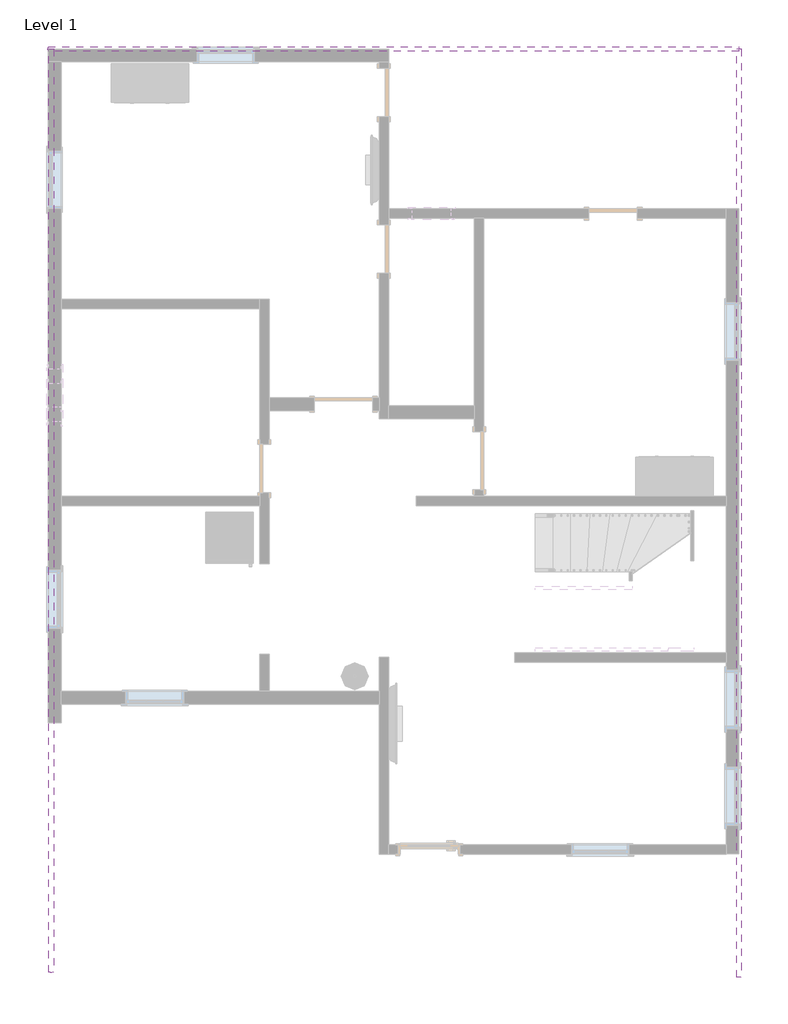
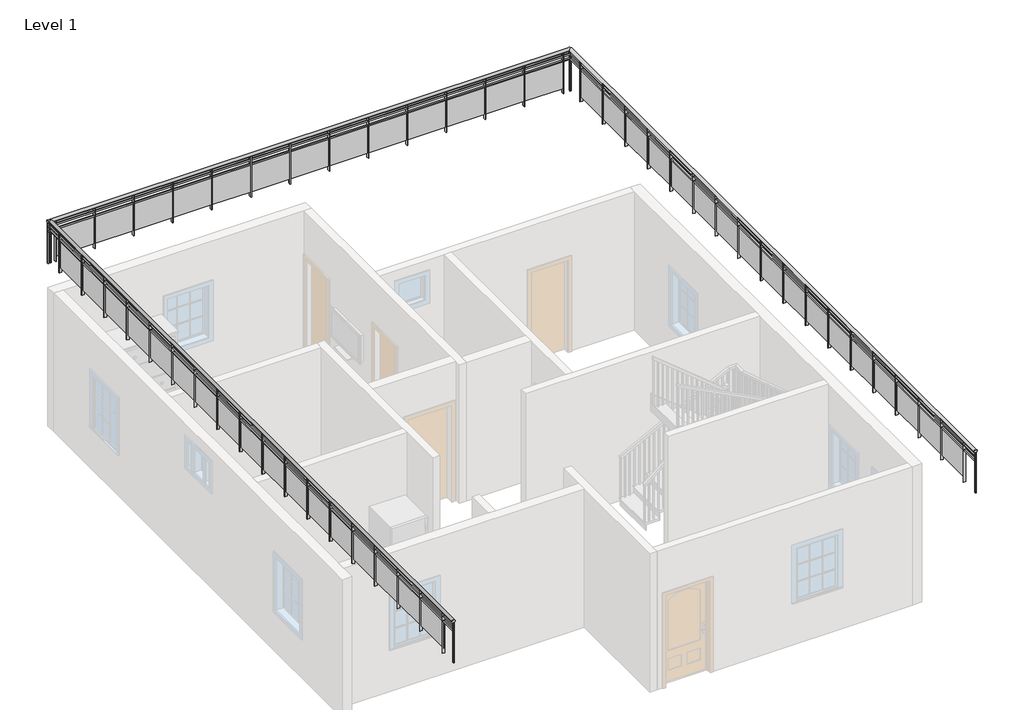
# One storey, part 3 of 4: 3 railings.
"""IFC4 building model written with IfcOpenShell, lengths in millimetres."""

from ifc_helpers import new_model, si_unit, point, frame, origin, place, context, project, spatial, polyline, ellipse_curve, trimmed, outline, extrude, element, save
from ifc_brep_helpers import plane_surface, extruded_surface, advanced_brep

model = new_model("IFC4")

# Units and contexts
model_context = context("Model", 3, world=origin())
ifc_project = project(units=[si_unit("LENGTHUNIT", "METRE", prefix="MILLI")], contexts=[model_context])

# Site, building, storey
site = spatial("IfcSite", under=ifc_project)
building = spatial("IfcBuilding", under=site)
storey = spatial("IfcBuildingStorey", under=building, Name="Level 1", Elevation=0.0)

# Railings
placement = place(None, origin())
element("IfcRailing", 1, ObjectType="Glass Panel - Bottom Fill", at=placement, inside=storey, context=model_context, shape_type="SolidModel", body=[
    advanced_brep(
    [(-12894.2866955, 15698.6787933, 4495.8), (-12970.4866955, 15698.6787933, 4495.8), (-12894.2866955, 1169.8787933, 4495.8), (-12970.4866955, 1169.8787933, 4495.8)],
    [
        (0, 1, ellipse_curve(frame((-12932.3866955, 15698.6787933, 4495.8), z_axis=(0.0, 1.0, 0.0), x_axis=(-1.0, 0.0, 0.0)), 38.1, 28.575)),
        (1, 0, ellipse_curve(frame((-12932.3866955, 15698.6787933, 4495.8), z_axis=(0.0, 1.0, 0.0), x_axis=(-1.0, 0.0, 0.0)), 38.1, 28.575)),
        (2, 3, ellipse_curve(frame((-12932.3866955, 1169.8787933, 4495.8), z_axis=(0.0, -1.0, 0.0), x_axis=(-1.0, 0.0, 0.0)), 38.1, 28.575)),
        (3, 2, ellipse_curve(frame((-12932.3866955, 1169.8787933, 4495.8), z_axis=(0.0, -1.0, 0.0), x_axis=(-1.0, 0.0, 0.0)), 38.1, 28.575)),
        (0, 2),
        (3, 1),
    ],
    [
        plane_surface(frame((-12932.3866955, 15698.6787933, 4495.8), z_axis=(0.0, 1.0, 0.0), x_axis=(0.0, 0.0, -1.0))),
        plane_surface(frame((-12932.3866955, 1169.8787933, 4495.8), z_axis=(0.0, -1.0, 0.0), x_axis=(0.0, 0.0, -1.0))),
        extruded_surface(trimmed(ellipse_curve(frame((-12932.3866955, 1169.8787933, 4495.8), z_axis=(0.0, 1.0, 0.0), x_axis=(-1.0, 0.0, 0.0)), 38.1, 28.575), [point((-12894.2866955, 1169.8787933, 4495.8))], [point((-12970.4866955, 1169.8787933, 4495.8))], True, "CARTESIAN"), (0.0, 14528.8, 0.0), 14528.8),
        extruded_surface(trimmed(ellipse_curve(frame((-12932.3866955, 1169.8787933, 4495.8), z_axis=(0.0, 1.0, 0.0), x_axis=(-1.0, 0.0, 0.0)), 38.1, 28.575), [point((-12970.4866955, 1169.8787933, 4495.8))], [point((-12894.2866955, 1169.8787933, 4495.8))], True, "CARTESIAN"), (0.0, 14528.8, 0.0), 14528.8),
    ],
    [
        (0, [[1, 2]]),
        (1, [[3, 4]]),
        (2, [[-1, 5, -4, 6]]),
        (3, [[-2, -6, -3, -5]]),
    ],
),
    extrude(outline(polyline([(-12945.0866955, 15698.6787933), (-12919.6866955, 15698.6787933), (-12919.6866955, 1169.8787933), (-12945.0866955, 1169.8787933), (-12945.0866955, 15698.6787933)])), frame((0.0, 0.0, 4381.5), z_axis=(0.0, 0.0, 1.0), x_axis=(1.0, 0.0, 0.0)), (0.0, 0.0, 1.0), 25.4),
    extrude(outline(polyline([(-12945.0866955, 15698.6787933), (-12919.6866955, 15698.6787933), (-12919.6866955, 1169.8787933), (-12945.0866955, 1169.8787933), (-12945.0866955, 15698.6787933)])), frame((0.0, 0.0, 4279.9), z_axis=(0.0, 0.0, 1.0), x_axis=(1.0, 0.0, 0.0)), (0.0, 0.0, 1.0), 25.4),
    extrude(outline(polyline([(-12957.7866955, 1531.8287933), (-12906.9866955, 1531.8287933), (-12906.9866955, 1519.1287933), (-12957.7866955, 1519.1287933), (-12957.7866955, 1531.8287933)])), frame((0.0, 0.0, 3581.4), z_axis=(0.0, 0.0, 1.0), x_axis=(1.0, 0.0, 0.0)), (0.0, 0.0, 1.0), 885.6788223),
    extrude(outline(polyline([(-12925.8515385, 2338.2787933), (-12925.8515385, 1525.4787933), (-12932.2015385, 1525.4787933), (-12932.2015385, 2338.2787933), (-12925.8515385, 2338.2787933)])), frame((0.0, 0.0, 3683.0), z_axis=(0.0, 0.0, 1.0), x_axis=(1.0, 0.0, 0.0)), (0.0, 0.0, 1.0), 596.9),
    extrude(outline(polyline([(-12957.7866955, 2344.6287933), (-12906.9866955, 2344.6287933), (-12906.9866955, 2331.9287933), (-12957.7866955, 2331.9287933), (-12957.7866955, 2344.6287933)])), frame((0.0, 0.0, 3581.4), z_axis=(0.0, 0.0, 1.0), x_axis=(1.0, 0.0, 0.0)), (0.0, 0.0, 1.0), 885.6788223),
    extrude(outline(polyline([(-12925.8515385, 3151.0787933), (-12925.8515385, 2338.2787933), (-12932.2015385, 2338.2787933), (-12932.2015385, 3151.0787933), (-12925.8515385, 3151.0787933)])), frame((0.0, 0.0, 3683.0), z_axis=(0.0, 0.0, 1.0), x_axis=(1.0, 0.0, 0.0)), (0.0, 0.0, 1.0), 596.9),
    extrude(outline(polyline([(-12957.7866955, 3157.4287933), (-12906.9866955, 3157.4287933), (-12906.9866955, 3144.7287933), (-12957.7866955, 3144.7287933), (-12957.7866955, 3157.4287933)])), frame((0.0, 0.0, 3581.4), z_axis=(0.0, 0.0, 1.0), x_axis=(1.0, 0.0, 0.0)), (0.0, 0.0, 1.0), 885.6788223),
    extrude(outline(polyline([(-12925.8515385, 3963.8787933), (-12925.8515385, 3151.0787933), (-12932.2015385, 3151.0787933), (-12932.2015385, 3963.8787933), (-12925.8515385, 3963.8787933)])), frame((0.0, 0.0, 3683.0), z_axis=(0.0, 0.0, 1.0), x_axis=(1.0, 0.0, 0.0)), (0.0, 0.0, 1.0), 596.9),
    extrude(outline(polyline([(-12957.7866955, 3970.2287933), (-12906.9866955, 3970.2287933), (-12906.9866955, 3957.5287933), (-12957.7866955, 3957.5287933), (-12957.7866955, 3970.2287933)])), frame((0.0, 0.0, 3581.4), z_axis=(0.0, 0.0, 1.0), x_axis=(1.0, 0.0, 0.0)), (0.0, 0.0, 1.0), 885.6788223),
    extrude(outline(polyline([(-12925.8515385, 4776.6787933), (-12925.8515385, 3963.8787933), (-12932.2015385, 3963.8787933), (-12932.2015385, 4776.6787933), (-12925.8515385, 4776.6787933)])), frame((0.0, 0.0, 3683.0), z_axis=(0.0, 0.0, 1.0), x_axis=(1.0, 0.0, 0.0)), (0.0, 0.0, 1.0), 596.9),
    extrude(outline(polyline([(-12957.7866955, 4783.0287933), (-12906.9866955, 4783.0287933), (-12906.9866955, 4770.3287933), (-12957.7866955, 4770.3287933), (-12957.7866955, 4783.0287933)])), frame((0.0, 0.0, 3581.4), z_axis=(0.0, 0.0, 1.0), x_axis=(1.0, 0.0, 0.0)), (0.0, 0.0, 1.0), 885.6788223),
    extrude(outline(polyline([(-12925.8515385, 5589.4787933), (-12925.8515385, 4776.6787933), (-12932.2015385, 4776.6787933), (-12932.2015385, 5589.4787933), (-12925.8515385, 5589.4787933)])), frame((0.0, 0.0, 3683.0), z_axis=(0.0, 0.0, 1.0), x_axis=(1.0, 0.0, 0.0)), (0.0, 0.0, 1.0), 596.9),
    extrude(outline(polyline([(-12957.7866955, 5595.8287933), (-12906.9866955, 5595.8287933), (-12906.9866955, 5583.1287933), (-12957.7866955, 5583.1287933), (-12957.7866955, 5595.8287933)])), frame((0.0, 0.0, 3581.4), z_axis=(0.0, 0.0, 1.0), x_axis=(1.0, 0.0, 0.0)), (0.0, 0.0, 1.0), 885.6788223),
    extrude(outline(polyline([(-12925.8515385, 6402.2787933), (-12925.8515385, 5589.4787933), (-12932.2015385, 5589.4787933), (-12932.2015385, 6402.2787933), (-12925.8515385, 6402.2787933)])), frame((0.0, 0.0, 3683.0), z_axis=(0.0, 0.0, 1.0), x_axis=(1.0, 0.0, 0.0)), (0.0, 0.0, 1.0), 596.9),
    extrude(outline(polyline([(-12957.7866955, 6408.6287933), (-12906.9866955, 6408.6287933), (-12906.9866955, 6395.9287933), (-12957.7866955, 6395.9287933), (-12957.7866955, 6408.6287933)])), frame((0.0, 0.0, 3581.4), z_axis=(0.0, 0.0, 1.0), x_axis=(1.0, 0.0, 0.0)), (0.0, 0.0, 1.0), 885.6788223),
    extrude(outline(polyline([(-12925.8515385, 7215.0787933), (-12925.8515385, 6402.2787933), (-12932.2015385, 6402.2787933), (-12932.2015385, 7215.0787933), (-12925.8515385, 7215.0787933)])), frame((0.0, 0.0, 3683.0), z_axis=(0.0, 0.0, 1.0), x_axis=(1.0, 0.0, 0.0)), (0.0, 0.0, 1.0), 596.9),
    extrude(outline(polyline([(-12957.7866955, 7221.4287933), (-12906.9866955, 7221.4287933), (-12906.9866955, 7208.7287933), (-12957.7866955, 7208.7287933), (-12957.7866955, 7221.4287933)])), frame((0.0, 0.0, 3581.4), z_axis=(0.0, 0.0, 1.0), x_axis=(1.0, 0.0, 0.0)), (0.0, 0.0, 1.0), 885.6788223),
    extrude(outline(polyline([(-12925.8515385, 8027.8787933), (-12925.8515385, 7215.0787933), (-12932.2015385, 7215.0787933), (-12932.2015385, 8027.8787933), (-12925.8515385, 8027.8787933)])), frame((0.0, 0.0, 3683.0), z_axis=(0.0, 0.0, 1.0), x_axis=(1.0, 0.0, 0.0)), (0.0, 0.0, 1.0), 596.9),
    extrude(outline(polyline([(-12957.7866955, 8034.2287933), (-12906.9866955, 8034.2287933), (-12906.9866955, 8021.5287933), (-12957.7866955, 8021.5287933), (-12957.7866955, 8034.2287933)])), frame((0.0, 0.0, 3581.4), z_axis=(0.0, 0.0, 1.0), x_axis=(1.0, 0.0, 0.0)), (0.0, 0.0, 1.0), 885.6788223),
    extrude(outline(polyline([(-12925.8515385, 8840.6787933), (-12925.8515385, 8027.8787933), (-12932.2015385, 8027.8787933), (-12932.2015385, 8840.6787933), (-12925.8515385, 8840.6787933)])), frame((0.0, 0.0, 3683.0), z_axis=(0.0, 0.0, 1.0), x_axis=(1.0, 0.0, 0.0)), (0.0, 0.0, 1.0), 596.9),
    extrude(outline(polyline([(-12957.7866955, 8847.0287933), (-12906.9866955, 8847.0287933), (-12906.9866955, 8834.3287933), (-12957.7866955, 8834.3287933), (-12957.7866955, 8847.0287933)])), frame((0.0, 0.0, 3581.4), z_axis=(0.0, 0.0, 1.0), x_axis=(1.0, 0.0, 0.0)), (0.0, 0.0, 1.0), 885.6788223),
    extrude(outline(polyline([(-12925.8515385, 9653.4787933), (-12925.8515385, 8840.6787933), (-12932.2015385, 8840.6787933), (-12932.2015385, 9653.4787933), (-12925.8515385, 9653.4787933)])), frame((0.0, 0.0, 3683.0), z_axis=(0.0, 0.0, 1.0), x_axis=(1.0, 0.0, 0.0)), (0.0, 0.0, 1.0), 596.9),
    extrude(outline(polyline([(-12957.7866955, 9659.8287933), (-12906.9866955, 9659.8287933), (-12906.9866955, 9647.1287933), (-12957.7866955, 9647.1287933), (-12957.7866955, 9659.8287933)])), frame((0.0, 0.0, 3581.4), z_axis=(0.0, 0.0, 1.0), x_axis=(1.0, 0.0, 0.0)), (0.0, 0.0, 1.0), 885.6788223),
    extrude(outline(polyline([(-12925.8515385, 10466.2787933), (-12925.8515385, 9653.4787933), (-12932.2015385, 9653.4787933), (-12932.2015385, 10466.2787933), (-12925.8515385, 10466.2787933)])), frame((0.0, 0.0, 3683.0), z_axis=(0.0, 0.0, 1.0), x_axis=(1.0, 0.0, 0.0)), (0.0, 0.0, 1.0), 596.9),
    extrude(outline(polyline([(-12957.7866955, 10472.6287933), (-12906.9866955, 10472.6287933), (-12906.9866955, 10459.9287933), (-12957.7866955, 10459.9287933), (-12957.7866955, 10472.6287933)])), frame((0.0, 0.0, 3581.4), z_axis=(0.0, 0.0, 1.0), x_axis=(1.0, 0.0, 0.0)), (0.0, 0.0, 1.0), 885.6788223),
    extrude(outline(polyline([(-12925.8515385, 11279.0787933), (-12925.8515385, 10466.2787933), (-12932.2015385, 10466.2787933), (-12932.2015385, 11279.0787933), (-12925.8515385, 11279.0787933)])), frame((0.0, 0.0, 3683.0), z_axis=(0.0, 0.0, 1.0), x_axis=(1.0, 0.0, 0.0)), (0.0, 0.0, 1.0), 596.9),
    extrude(outline(polyline([(-12957.7866955, 11285.4287933), (-12906.9866955, 11285.4287933), (-12906.9866955, 11272.7287933), (-12957.7866955, 11272.7287933), (-12957.7866955, 11285.4287933)])), frame((0.0, 0.0, 3581.4), z_axis=(0.0, 0.0, 1.0), x_axis=(1.0, 0.0, 0.0)), (0.0, 0.0, 1.0), 885.6788223),
    extrude(outline(polyline([(-12925.8515385, 12091.8787933), (-12925.8515385, 11279.0787933), (-12932.2015385, 11279.0787933), (-12932.2015385, 12091.8787933), (-12925.8515385, 12091.8787933)])), frame((0.0, 0.0, 3683.0), z_axis=(0.0, 0.0, 1.0), x_axis=(1.0, 0.0, 0.0)), (0.0, 0.0, 1.0), 596.9),
    extrude(outline(polyline([(-12957.7866955, 12098.2287933), (-12906.9866955, 12098.2287933), (-12906.9866955, 12085.5287933), (-12957.7866955, 12085.5287933), (-12957.7866955, 12098.2287933)])), frame((0.0, 0.0, 3581.4), z_axis=(0.0, 0.0, 1.0), x_axis=(1.0, 0.0, 0.0)), (0.0, 0.0, 1.0), 885.6788223),
    extrude(outline(polyline([(-12925.8515385, 12904.6787933), (-12925.8515385, 12091.8787933), (-12932.2015385, 12091.8787933), (-12932.2015385, 12904.6787933), (-12925.8515385, 12904.6787933)])), frame((0.0, 0.0, 3683.0), z_axis=(0.0, 0.0, 1.0), x_axis=(1.0, 0.0, 0.0)), (0.0, 0.0, 1.0), 596.9),
    extrude(outline(polyline([(-12957.7866955, 12911.0287933), (-12906.9866955, 12911.0287933), (-12906.9866955, 12898.3287933), (-12957.7866955, 12898.3287933), (-12957.7866955, 12911.0287933)])), frame((0.0, 0.0, 3581.4), z_axis=(0.0, 0.0, 1.0), x_axis=(1.0, 0.0, 0.0)), (0.0, 0.0, 1.0), 885.6788223),
    extrude(outline(polyline([(-12925.8515385, 13717.4787933), (-12925.8515385, 12904.6787933), (-12932.2015385, 12904.6787933), (-12932.2015385, 13717.4787933), (-12925.8515385, 13717.4787933)])), frame((0.0, 0.0, 3683.0), z_axis=(0.0, 0.0, 1.0), x_axis=(1.0, 0.0, 0.0)), (0.0, 0.0, 1.0), 596.9),
    extrude(outline(polyline([(-12957.7866955, 13723.8287933), (-12906.9866955, 13723.8287933), (-12906.9866955, 13711.1287933), (-12957.7866955, 13711.1287933), (-12957.7866955, 13723.8287933)])), frame((0.0, 0.0, 3581.4), z_axis=(0.0, 0.0, 1.0), x_axis=(1.0, 0.0, 0.0)), (0.0, 0.0, 1.0), 885.6788223),
    extrude(outline(polyline([(-12925.8515385, 14530.2787933), (-12925.8515385, 13717.4787933), (-12932.2015385, 13717.4787933), (-12932.2015385, 14530.2787933), (-12925.8515385, 14530.2787933)])), frame((0.0, 0.0, 3683.0), z_axis=(0.0, 0.0, 1.0), x_axis=(1.0, 0.0, 0.0)), (0.0, 0.0, 1.0), 596.9),
    extrude(outline(polyline([(-12957.7866955, 14536.6287933), (-12906.9866955, 14536.6287933), (-12906.9866955, 14523.9287933), (-12957.7866955, 14523.9287933), (-12957.7866955, 14536.6287933)])), frame((0.0, 0.0, 3581.4), z_axis=(0.0, 0.0, 1.0), x_axis=(1.0, 0.0, 0.0)), (0.0, 0.0, 1.0), 885.6788223),
    extrude(outline(polyline([(-12925.8515385, 15343.0787933), (-12925.8515385, 14530.2787933), (-12932.2015385, 14530.2787933), (-12932.2015385, 15343.0787933), (-12925.8515385, 15343.0787933)])), frame((0.0, 0.0, 3683.0), z_axis=(0.0, 0.0, 1.0), x_axis=(1.0, 0.0, 0.0)), (0.0, 0.0, 1.0), 596.9),
    extrude(outline(polyline([(-12957.7866955, 15349.4287933), (-12906.9866955, 15349.4287933), (-12906.9866955, 15336.7287933), (-12957.7866955, 15336.7287933), (-12957.7866955, 15349.4287933)])), frame((0.0, 0.0, 3581.4), z_axis=(0.0, 0.0, 1.0), x_axis=(1.0, 0.0, 0.0)), (0.0, 0.0, 1.0), 885.6788223),
    extrude(outline(polyline([(-12941.9116955, 1182.5787933), (-12922.8616955, 1182.5787933), (-12922.8616955, 1163.5287933), (-12941.9116955, 1163.5287933), (-12941.9116955, 1182.5787933)])), frame((0.0, 0.0, 3581.4), z_axis=(0.0, 0.0, 1.0), x_axis=(1.0, 0.0, 0.0)), (0.0, 0.0, 1.0), 885.6788223),
    extrude(outline(polyline([(-12941.9116955, 15705.0287933), (-12922.8616955, 15705.0287933), (-12922.8616955, 15685.9787933), (-12941.9116955, 15685.9787933), (-12941.9116955, 15705.0287933)])), frame((0.0, 0.0, 3581.4), z_axis=(0.0, 0.0, 1.0), x_axis=(1.0, 0.0, 0.0)), (0.0, 0.0, 1.0), 885.6788223),
])
element("IfcRailing", 2, ObjectType="Glass Panel - Bottom Fill", at=placement, inside=storey, context=model_context, shape_type="SolidModel", body=[
    advanced_brep(
    [(-2150.0866955, 1093.6787933, 4495.8), (-2073.8866955, 1093.6787933, 4495.8), (-2150.0866955, 15698.6787933, 4495.8), (-2073.8866955, 15698.6787933, 4495.8)],
    [
        (0, 1, ellipse_curve(frame((-2111.9866955, 1093.6787933, 4495.8), z_axis=(0.0, -1.0, 0.0), x_axis=(1.0, 0.0, 0.0)), 38.1, 28.575)),
        (1, 0, ellipse_curve(frame((-2111.9866955, 1093.6787933, 4495.8), z_axis=(0.0, -1.0, 0.0), x_axis=(1.0, 0.0, 0.0)), 38.1, 28.575)),
        (2, 3, ellipse_curve(frame((-2111.9866955, 15698.6787933, 4495.8), z_axis=(0.0, 1.0, 0.0), x_axis=(1.0, 0.0, 0.0)), 38.1, 28.575)),
        (3, 2, ellipse_curve(frame((-2111.9866955, 15698.6787933, 4495.8), z_axis=(0.0, 1.0, 0.0), x_axis=(1.0, 0.0, 0.0)), 38.1, 28.575)),
        (0, 2),
        (3, 1),
    ],
    [
        plane_surface(frame((-2111.9866955, 1093.6787933, 4495.8), z_axis=(0.0, -1.0, 0.0), x_axis=(0.0, 0.0, 1.0))),
        plane_surface(frame((-2111.9866955, 15698.6787933, 4495.8), z_axis=(0.0, 1.0, 0.0), x_axis=(0.0, 0.0, 1.0))),
        extruded_surface(trimmed(ellipse_curve(frame((-2111.9866955, 15698.6787933, 4495.8), z_axis=(0.0, -1.0, 0.0), x_axis=(1.0, 0.0, 0.0)), 38.1, 28.575), [point((-2150.0866955, 15698.6787933, 4495.8))], [point((-2073.8866955, 15698.6787933, 4495.8))], True, "CARTESIAN"), (0.0, -14605.0, 0.0), 14605.0),
        extruded_surface(trimmed(ellipse_curve(frame((-2111.9866955, 15698.6787933, 4495.8), z_axis=(0.0, -1.0, 0.0), x_axis=(1.0, 0.0, 0.0)), 38.1, 28.575), [point((-2073.8866955, 15698.6787933, 4495.8))], [point((-2150.0866955, 15698.6787933, 4495.8))], True, "CARTESIAN"), (0.0, -14605.0, 0.0), 14605.0),
    ],
    [
        (0, [[1, 2]]),
        (1, [[3, 4]]),
        (2, [[-1, 5, -4, 6]]),
        (3, [[-2, -6, -3, -5]]),
    ],
),
    extrude(outline(polyline([(-2099.2866955, 1093.6787933), (-2124.6866955, 1093.6787933), (-2124.6866955, 15698.6787933), (-2099.2866955, 15698.6787933), (-2099.2866955, 1093.6787933)])), frame((0.0, 0.0, 4381.5), z_axis=(0.0, 0.0, 1.0), x_axis=(1.0, 0.0, 0.0)), (0.0, 0.0, 1.0), 25.4),
    extrude(outline(polyline([(-2099.2866955, 1093.6787933), (-2124.6866955, 1093.6787933), (-2124.6866955, 15698.6787933), (-2099.2866955, 15698.6787933), (-2099.2866955, 1093.6787933)])), frame((0.0, 0.0, 4279.9), z_axis=(0.0, 0.0, 1.0), x_axis=(1.0, 0.0, 0.0)), (0.0, 0.0, 1.0), 25.4),
    extrude(outline(polyline([(-2086.5866955, 15298.6287933), (-2137.3866955, 15298.6287933), (-2137.3866955, 15311.3287933), (-2086.5866955, 15311.3287933), (-2086.5866955, 15298.6287933)])), frame((0.0, 0.0, 3581.4), z_axis=(0.0, 0.0, 1.0), x_axis=(1.0, 0.0, 0.0)), (0.0, 0.0, 1.0), 885.6788223),
    extrude(outline(polyline([(-2118.5218525, 14492.1787933), (-2118.5218525, 15304.9787933), (-2112.1718525, 15304.9787933), (-2112.1718525, 14492.1787933), (-2118.5218525, 14492.1787933)])), frame((0.0, 0.0, 3683.0), z_axis=(0.0, 0.0, 1.0), x_axis=(1.0, 0.0, 0.0)), (0.0, 0.0, 1.0), 596.9),
    extrude(outline(polyline([(-2086.5866955, 14485.8287933), (-2137.3866955, 14485.8287933), (-2137.3866955, 14498.5287933), (-2086.5866955, 14498.5287933), (-2086.5866955, 14485.8287933)])), frame((0.0, 0.0, 3581.4), z_axis=(0.0, 0.0, 1.0), x_axis=(1.0, 0.0, 0.0)), (0.0, 0.0, 1.0), 885.6788223),
    extrude(outline(polyline([(-2118.5218525, 13679.3787933), (-2118.5218525, 14492.1787933), (-2112.1718525, 14492.1787933), (-2112.1718525, 13679.3787933), (-2118.5218525, 13679.3787933)])), frame((0.0, 0.0, 3683.0), z_axis=(0.0, 0.0, 1.0), x_axis=(1.0, 0.0, 0.0)), (0.0, 0.0, 1.0), 596.9),
    extrude(outline(polyline([(-2086.5866955, 13673.0287933), (-2137.3866955, 13673.0287933), (-2137.3866955, 13685.7287933), (-2086.5866955, 13685.7287933), (-2086.5866955, 13673.0287933)])), frame((0.0, 0.0, 3581.4), z_axis=(0.0, 0.0, 1.0), x_axis=(1.0, 0.0, 0.0)), (0.0, 0.0, 1.0), 885.6788223),
    extrude(outline(polyline([(-2118.5218525, 12866.5787933), (-2118.5218525, 13679.3787933), (-2112.1718525, 13679.3787933), (-2112.1718525, 12866.5787933), (-2118.5218525, 12866.5787933)])), frame((0.0, 0.0, 3683.0), z_axis=(0.0, 0.0, 1.0), x_axis=(1.0, 0.0, 0.0)), (0.0, 0.0, 1.0), 596.9),
    extrude(outline(polyline([(-2086.5866955, 12860.2287933), (-2137.3866955, 12860.2287933), (-2137.3866955, 12872.9287933), (-2086.5866955, 12872.9287933), (-2086.5866955, 12860.2287933)])), frame((0.0, 0.0, 3581.4), z_axis=(0.0, 0.0, 1.0), x_axis=(1.0, 0.0, 0.0)), (0.0, 0.0, 1.0), 885.6788223),
    extrude(outline(polyline([(-2118.5218525, 12053.7787933), (-2118.5218525, 12866.5787933), (-2112.1718525, 12866.5787933), (-2112.1718525, 12053.7787933), (-2118.5218525, 12053.7787933)])), frame((0.0, 0.0, 3683.0), z_axis=(0.0, 0.0, 1.0), x_axis=(1.0, 0.0, 0.0)), (0.0, 0.0, 1.0), 596.9),
    extrude(outline(polyline([(-2086.5866955, 12047.4287933), (-2137.3866955, 12047.4287933), (-2137.3866955, 12060.1287933), (-2086.5866955, 12060.1287933), (-2086.5866955, 12047.4287933)])), frame((0.0, 0.0, 3581.4), z_axis=(0.0, 0.0, 1.0), x_axis=(1.0, 0.0, 0.0)), (0.0, 0.0, 1.0), 885.6788223),
    extrude(outline(polyline([(-2118.5218525, 11240.9787933), (-2118.5218525, 12053.7787933), (-2112.1718525, 12053.7787933), (-2112.1718525, 11240.9787933), (-2118.5218525, 11240.9787933)])), frame((0.0, 0.0, 3683.0), z_axis=(0.0, 0.0, 1.0), x_axis=(1.0, 0.0, 0.0)), (0.0, 0.0, 1.0), 596.9),
    extrude(outline(polyline([(-2086.5866955, 11234.6287933), (-2137.3866955, 11234.6287933), (-2137.3866955, 11247.3287933), (-2086.5866955, 11247.3287933), (-2086.5866955, 11234.6287933)])), frame((0.0, 0.0, 3581.4), z_axis=(0.0, 0.0, 1.0), x_axis=(1.0, 0.0, 0.0)), (0.0, 0.0, 1.0), 885.6788223),
    extrude(outline(polyline([(-2118.5218525, 10428.1787933), (-2118.5218525, 11240.9787933), (-2112.1718525, 11240.9787933), (-2112.1718525, 10428.1787933), (-2118.5218525, 10428.1787933)])), frame((0.0, 0.0, 3683.0), z_axis=(0.0, 0.0, 1.0), x_axis=(1.0, 0.0, 0.0)), (0.0, 0.0, 1.0), 596.9),
    extrude(outline(polyline([(-2086.5866955, 10421.8287933), (-2137.3866955, 10421.8287933), (-2137.3866955, 10434.5287933), (-2086.5866955, 10434.5287933), (-2086.5866955, 10421.8287933)])), frame((0.0, 0.0, 3581.4), z_axis=(0.0, 0.0, 1.0), x_axis=(1.0, 0.0, 0.0)), (0.0, 0.0, 1.0), 885.6788223),
    extrude(outline(polyline([(-2118.5218525, 9615.3787933), (-2118.5218525, 10428.1787933), (-2112.1718525, 10428.1787933), (-2112.1718525, 9615.3787933), (-2118.5218525, 9615.3787933)])), frame((0.0, 0.0, 3683.0), z_axis=(0.0, 0.0, 1.0), x_axis=(1.0, 0.0, 0.0)), (0.0, 0.0, 1.0), 596.9),
    extrude(outline(polyline([(-2086.5866955, 9609.0287933), (-2137.3866955, 9609.0287933), (-2137.3866955, 9621.7287933), (-2086.5866955, 9621.7287933), (-2086.5866955, 9609.0287933)])), frame((0.0, 0.0, 3581.4), z_axis=(0.0, 0.0, 1.0), x_axis=(1.0, 0.0, 0.0)), (0.0, 0.0, 1.0), 885.6788223),
    extrude(outline(polyline([(-2118.5218525, 8802.5787933), (-2118.5218525, 9615.3787933), (-2112.1718525, 9615.3787933), (-2112.1718525, 8802.5787933), (-2118.5218525, 8802.5787933)])), frame((0.0, 0.0, 3683.0), z_axis=(0.0, 0.0, 1.0), x_axis=(1.0, 0.0, 0.0)), (0.0, 0.0, 1.0), 596.9),
    extrude(outline(polyline([(-2086.5866955, 8796.2287933), (-2137.3866955, 8796.2287933), (-2137.3866955, 8808.9287933), (-2086.5866955, 8808.9287933), (-2086.5866955, 8796.2287933)])), frame((0.0, 0.0, 3581.4), z_axis=(0.0, 0.0, 1.0), x_axis=(1.0, 0.0, 0.0)), (0.0, 0.0, 1.0), 885.6788223),
    extrude(outline(polyline([(-2118.5218525, 7989.7787933), (-2118.5218525, 8802.5787933), (-2112.1718525, 8802.5787933), (-2112.1718525, 7989.7787933), (-2118.5218525, 7989.7787933)])), frame((0.0, 0.0, 3683.0), z_axis=(0.0, 0.0, 1.0), x_axis=(1.0, 0.0, 0.0)), (0.0, 0.0, 1.0), 596.9),
    extrude(outline(polyline([(-2086.5866955, 7983.4287933), (-2137.3866955, 7983.4287933), (-2137.3866955, 7996.1287933), (-2086.5866955, 7996.1287933), (-2086.5866955, 7983.4287933)])), frame((0.0, 0.0, 3581.4), z_axis=(0.0, 0.0, 1.0), x_axis=(1.0, 0.0, 0.0)), (0.0, 0.0, 1.0), 885.6788223),
    extrude(outline(polyline([(-2118.5218525, 7176.9787933), (-2118.5218525, 7989.7787933), (-2112.1718525, 7989.7787933), (-2112.1718525, 7176.9787933), (-2118.5218525, 7176.9787933)])), frame((0.0, 0.0, 3683.0), z_axis=(0.0, 0.0, 1.0), x_axis=(1.0, 0.0, 0.0)), (0.0, 0.0, 1.0), 596.9),
    extrude(outline(polyline([(-2086.5866955, 7170.6287933), (-2137.3866955, 7170.6287933), (-2137.3866955, 7183.3287933), (-2086.5866955, 7183.3287933), (-2086.5866955, 7170.6287933)])), frame((0.0, 0.0, 3581.4), z_axis=(0.0, 0.0, 1.0), x_axis=(1.0, 0.0, 0.0)), (0.0, 0.0, 1.0), 885.6788223),
    extrude(outline(polyline([(-2118.5218525, 6364.1787933), (-2118.5218525, 7176.9787933), (-2112.1718525, 7176.9787933), (-2112.1718525, 6364.1787933), (-2118.5218525, 6364.1787933)])), frame((0.0, 0.0, 3683.0), z_axis=(0.0, 0.0, 1.0), x_axis=(1.0, 0.0, 0.0)), (0.0, 0.0, 1.0), 596.9),
    extrude(outline(polyline([(-2086.5866955, 6357.8287933), (-2137.3866955, 6357.8287933), (-2137.3866955, 6370.5287933), (-2086.5866955, 6370.5287933), (-2086.5866955, 6357.8287933)])), frame((0.0, 0.0, 3581.4), z_axis=(0.0, 0.0, 1.0), x_axis=(1.0, 0.0, 0.0)), (0.0, 0.0, 1.0), 885.6788223),
    extrude(outline(polyline([(-2118.5218525, 5551.3787933), (-2118.5218525, 6364.1787933), (-2112.1718525, 6364.1787933), (-2112.1718525, 5551.3787933), (-2118.5218525, 5551.3787933)])), frame((0.0, 0.0, 3683.0), z_axis=(0.0, 0.0, 1.0), x_axis=(1.0, 0.0, 0.0)), (0.0, 0.0, 1.0), 596.9),
    extrude(outline(polyline([(-2086.5866955, 5545.0287933), (-2137.3866955, 5545.0287933), (-2137.3866955, 5557.7287933), (-2086.5866955, 5557.7287933), (-2086.5866955, 5545.0287933)])), frame((0.0, 0.0, 3581.4), z_axis=(0.0, 0.0, 1.0), x_axis=(1.0, 0.0, 0.0)), (0.0, 0.0, 1.0), 885.6788223),
    extrude(outline(polyline([(-2118.5218525, 4738.5787933), (-2118.5218525, 5551.3787933), (-2112.1718525, 5551.3787933), (-2112.1718525, 4738.5787933), (-2118.5218525, 4738.5787933)])), frame((0.0, 0.0, 3683.0), z_axis=(0.0, 0.0, 1.0), x_axis=(1.0, 0.0, 0.0)), (0.0, 0.0, 1.0), 596.9),
    extrude(outline(polyline([(-2086.5866955, 4732.2287933), (-2137.3866955, 4732.2287933), (-2137.3866955, 4744.9287933), (-2086.5866955, 4744.9287933), (-2086.5866955, 4732.2287933)])), frame((0.0, 0.0, 3581.4), z_axis=(0.0, 0.0, 1.0), x_axis=(1.0, 0.0, 0.0)), (0.0, 0.0, 1.0), 885.6788223),
    extrude(outline(polyline([(-2118.5218525, 3925.7787933), (-2118.5218525, 4738.5787933), (-2112.1718525, 4738.5787933), (-2112.1718525, 3925.7787933), (-2118.5218525, 3925.7787933)])), frame((0.0, 0.0, 3683.0), z_axis=(0.0, 0.0, 1.0), x_axis=(1.0, 0.0, 0.0)), (0.0, 0.0, 1.0), 596.9),
    extrude(outline(polyline([(-2086.5866955, 3919.4287933), (-2137.3866955, 3919.4287933), (-2137.3866955, 3932.1287933), (-2086.5866955, 3932.1287933), (-2086.5866955, 3919.4287933)])), frame((0.0, 0.0, 3581.4), z_axis=(0.0, 0.0, 1.0), x_axis=(1.0, 0.0, 0.0)), (0.0, 0.0, 1.0), 885.6788223),
    extrude(outline(polyline([(-2118.5218525, 3112.9787933), (-2118.5218525, 3925.7787933), (-2112.1718525, 3925.7787933), (-2112.1718525, 3112.9787933), (-2118.5218525, 3112.9787933)])), frame((0.0, 0.0, 3683.0), z_axis=(0.0, 0.0, 1.0), x_axis=(1.0, 0.0, 0.0)), (0.0, 0.0, 1.0), 596.9),
    extrude(outline(polyline([(-2086.5866955, 3106.6287933), (-2137.3866955, 3106.6287933), (-2137.3866955, 3119.3287933), (-2086.5866955, 3119.3287933), (-2086.5866955, 3106.6287933)])), frame((0.0, 0.0, 3581.4), z_axis=(0.0, 0.0, 1.0), x_axis=(1.0, 0.0, 0.0)), (0.0, 0.0, 1.0), 885.6788223),
    extrude(outline(polyline([(-2118.5218525, 2300.1787933), (-2118.5218525, 3112.9787933), (-2112.1718525, 3112.9787933), (-2112.1718525, 2300.1787933), (-2118.5218525, 2300.1787933)])), frame((0.0, 0.0, 3683.0), z_axis=(0.0, 0.0, 1.0), x_axis=(1.0, 0.0, 0.0)), (0.0, 0.0, 1.0), 596.9),
    extrude(outline(polyline([(-2086.5866955, 2293.8287933), (-2137.3866955, 2293.8287933), (-2137.3866955, 2306.5287933), (-2086.5866955, 2306.5287933), (-2086.5866955, 2293.8287933)])), frame((0.0, 0.0, 3581.4), z_axis=(0.0, 0.0, 1.0), x_axis=(1.0, 0.0, 0.0)), (0.0, 0.0, 1.0), 885.6788223),
    extrude(outline(polyline([(-2118.5218525, 1487.3787933), (-2118.5218525, 2300.1787933), (-2112.1718525, 2300.1787933), (-2112.1718525, 1487.3787933), (-2118.5218525, 1487.3787933)])), frame((0.0, 0.0, 3683.0), z_axis=(0.0, 0.0, 1.0), x_axis=(1.0, 0.0, 0.0)), (0.0, 0.0, 1.0), 596.9),
    extrude(outline(polyline([(-2086.5866955, 1481.0287933), (-2137.3866955, 1481.0287933), (-2137.3866955, 1493.7287933), (-2086.5866955, 1493.7287933), (-2086.5866955, 1481.0287933)])), frame((0.0, 0.0, 3581.4), z_axis=(0.0, 0.0, 1.0), x_axis=(1.0, 0.0, 0.0)), (0.0, 0.0, 1.0), 885.6788223),
    extrude(outline(polyline([(-2102.4616955, 15685.9787933), (-2121.5116955, 15685.9787933), (-2121.5116955, 15705.0287933), (-2102.4616955, 15705.0287933), (-2102.4616955, 15685.9787933)])), frame((0.0, 0.0, 3581.4), z_axis=(0.0, 0.0, 1.0), x_axis=(1.0, 0.0, 0.0)), (0.0, 0.0, 1.0), 885.6788223),
    extrude(outline(polyline([(-2102.4616955, 1087.3287933), (-2121.5116955, 1087.3287933), (-2121.5116955, 1106.3787933), (-2102.4616955, 1106.3787933), (-2102.4616955, 1087.3287933)])), frame((0.0, 0.0, 3581.4), z_axis=(0.0, 0.0, 1.0), x_axis=(1.0, 0.0, 0.0)), (0.0, 0.0, 1.0), 885.6788223),
])
element("IfcRailing", 3, ObjectType="Glass Panel - Bottom Fill", at=placement, inside=storey, context=model_context, shape_type="SolidModel", body=[
    advanced_brep(
    [(-2111.9866955, 15660.5787933, 4495.8), (-2111.9866955, 15736.7787933, 4495.8), (-12983.1866955, 15660.5787933, 4495.8), (-12983.1866955, 15736.7787933, 4495.8)],
    [
        (0, 1, ellipse_curve(frame((-2111.9866955, 15698.6787933, 4495.8), z_axis=(1.0, 0.0, 0.0), x_axis=(0.0, 1.0, 0.0)), 38.1, 28.575)),
        (1, 0, ellipse_curve(frame((-2111.9866955, 15698.6787933, 4495.8), z_axis=(1.0, 0.0, 0.0), x_axis=(0.0, 1.0, 0.0)), 38.1, 28.575)),
        (2, 3, ellipse_curve(frame((-12983.1866955, 15698.6787933, 4495.8), z_axis=(-1.0, 0.0, 0.0), x_axis=(0.0, 1.0, 0.0)), 38.1, 28.575)),
        (3, 2, ellipse_curve(frame((-12983.1866955, 15698.6787933, 4495.8), z_axis=(-1.0, 0.0, 0.0), x_axis=(0.0, 1.0, 0.0)), 38.1, 28.575)),
        (0, 2),
        (3, 1),
    ],
    [
        plane_surface(frame((-2111.9866955, 15698.6787933, 4495.8), z_axis=(1.0, 0.0, 0.0), x_axis=(0.0, -1.0, 0.0))),
        plane_surface(frame((-12983.1866955, 15698.6787933, 4495.8), z_axis=(-1.0, 0.0, 0.0), x_axis=(0.0, -1.0, 0.0))),
        extruded_surface(trimmed(ellipse_curve(frame((-12983.1866955, 15698.6787933, 4495.8), z_axis=(1.0, 0.0, 0.0), x_axis=(0.0, 1.0, 0.0)), 38.1, 28.575), [point((-12983.1866955, 15660.5787933, 4495.8))], [point((-12983.1866955, 15736.7787933, 4495.8))], True, "CARTESIAN"), (10871.2, 0.0, 0.0), 10871.2),
        extruded_surface(trimmed(ellipse_curve(frame((-12983.1866955, 15698.6787933, 4495.8), z_axis=(1.0, 0.0, 0.0), x_axis=(0.0, 1.0, 0.0)), 38.1, 28.575), [point((-12983.1866955, 15736.7787933, 4495.8))], [point((-12983.1866955, 15660.5787933, 4495.8))], True, "CARTESIAN"), (10871.2, 0.0, 0.0), 10871.2),
    ],
    [
        (0, [[1, 2]]),
        (1, [[3, 4]]),
        (2, [[-1, 5, -4, 6]]),
        (3, [[-2, -6, -3, -5]]),
    ],
),
    extrude(outline(polyline([(-2111.9866955, 15711.3787933), (-2111.9866955, 15685.9787933), (-12983.1866955, 15685.9787933), (-12983.1866955, 15711.3787933), (-2111.9866955, 15711.3787933)])), frame((0.0, 0.0, 4381.5), z_axis=(0.0, 0.0, 1.0), x_axis=(1.0, 0.0, 0.0)), (0.0, 0.0, 1.0), 25.4),
    extrude(outline(polyline([(-2111.9866955, 15711.3787933), (-2111.9866955, 15685.9787933), (-12983.1866955, 15685.9787933), (-12983.1866955, 15711.3787933), (-2111.9866955, 15711.3787933)])), frame((0.0, 0.0, 4279.9), z_axis=(0.0, 0.0, 1.0), x_axis=(1.0, 0.0, 0.0)), (0.0, 0.0, 1.0), 25.4),
    extrude(outline(polyline([(-12824.4366955, 15724.0787933), (-12824.4366955, 15673.2787933), (-12837.1366955, 15673.2787933), (-12837.1366955, 15724.0787933), (-12824.4366955, 15724.0787933)])), frame((0.0, 0.0, 3581.4), z_axis=(0.0, 0.0, 1.0), x_axis=(1.0, 0.0, 0.0)), (0.0, 0.0, 1.0), 885.6788223),
    extrude(outline(polyline([(-12017.9866955, 15692.1436363), (-12830.7866955, 15692.1436363), (-12830.7866955, 15698.4936363), (-12017.9866955, 15698.4936363), (-12017.9866955, 15692.1436363)])), frame((0.0, 0.0, 3683.0), z_axis=(0.0, 0.0, 1.0), x_axis=(1.0, 0.0, 0.0)), (0.0, 0.0, 1.0), 596.9),
    extrude(outline(polyline([(-12011.6366955, 15724.0787933), (-12011.6366955, 15673.2787933), (-12024.3366955, 15673.2787933), (-12024.3366955, 15724.0787933), (-12011.6366955, 15724.0787933)])), frame((0.0, 0.0, 3581.4), z_axis=(0.0, 0.0, 1.0), x_axis=(1.0, 0.0, 0.0)), (0.0, 0.0, 1.0), 885.6788223),
    extrude(outline(polyline([(-11205.1866955, 15692.1436363), (-12017.9866955, 15692.1436363), (-12017.9866955, 15698.4936363), (-11205.1866955, 15698.4936363), (-11205.1866955, 15692.1436363)])), frame((0.0, 0.0, 3683.0), z_axis=(0.0, 0.0, 1.0), x_axis=(1.0, 0.0, 0.0)), (0.0, 0.0, 1.0), 596.9),
    extrude(outline(polyline([(-11198.8366955, 15724.0787933), (-11198.8366955, 15673.2787933), (-11211.5366955, 15673.2787933), (-11211.5366955, 15724.0787933), (-11198.8366955, 15724.0787933)])), frame((0.0, 0.0, 3581.4), z_axis=(0.0, 0.0, 1.0), x_axis=(1.0, 0.0, 0.0)), (0.0, 0.0, 1.0), 885.6788223),
    extrude(outline(polyline([(-10392.3866955, 15692.1436363), (-11205.1866955, 15692.1436363), (-11205.1866955, 15698.4936363), (-10392.3866955, 15698.4936363), (-10392.3866955, 15692.1436363)])), frame((0.0, 0.0, 3683.0), z_axis=(0.0, 0.0, 1.0), x_axis=(1.0, 0.0, 0.0)), (0.0, 0.0, 1.0), 596.9),
    extrude(outline(polyline([(-10386.0366955, 15724.0787933), (-10386.0366955, 15673.2787933), (-10398.7366955, 15673.2787933), (-10398.7366955, 15724.0787933), (-10386.0366955, 15724.0787933)])), frame((0.0, 0.0, 3581.4), z_axis=(0.0, 0.0, 1.0), x_axis=(1.0, 0.0, 0.0)), (0.0, 0.0, 1.0), 885.6788223),
    extrude(outline(polyline([(-9579.5866955, 15692.1436363), (-10392.3866955, 15692.1436363), (-10392.3866955, 15698.4936363), (-9579.5866955, 15698.4936363), (-9579.5866955, 15692.1436363)])), frame((0.0, 0.0, 3683.0), z_axis=(0.0, 0.0, 1.0), x_axis=(1.0, 0.0, 0.0)), (0.0, 0.0, 1.0), 596.9),
    extrude(outline(polyline([(-9573.2366955, 15724.0787933), (-9573.2366955, 15673.2787933), (-9585.9366955, 15673.2787933), (-9585.9366955, 15724.0787933), (-9573.2366955, 15724.0787933)])), frame((0.0, 0.0, 3581.4), z_axis=(0.0, 0.0, 1.0), x_axis=(1.0, 0.0, 0.0)), (0.0, 0.0, 1.0), 885.6788223),
    extrude(outline(polyline([(-8766.7866955, 15692.1436363), (-9579.5866955, 15692.1436363), (-9579.5866955, 15698.4936363), (-8766.7866955, 15698.4936363), (-8766.7866955, 15692.1436363)])), frame((0.0, 0.0, 3683.0), z_axis=(0.0, 0.0, 1.0), x_axis=(1.0, 0.0, 0.0)), (0.0, 0.0, 1.0), 596.9),
    extrude(outline(polyline([(-8760.4366955, 15724.0787933), (-8760.4366955, 15673.2787933), (-8773.1366955, 15673.2787933), (-8773.1366955, 15724.0787933), (-8760.4366955, 15724.0787933)])), frame((0.0, 0.0, 3581.4), z_axis=(0.0, 0.0, 1.0), x_axis=(1.0, 0.0, 0.0)), (0.0, 0.0, 1.0), 885.6788223),
    extrude(outline(polyline([(-7953.9866955, 15692.1436363), (-8766.7866955, 15692.1436363), (-8766.7866955, 15698.4936363), (-7953.9866955, 15698.4936363), (-7953.9866955, 15692.1436363)])), frame((0.0, 0.0, 3683.0), z_axis=(0.0, 0.0, 1.0), x_axis=(1.0, 0.0, 0.0)), (0.0, 0.0, 1.0), 596.9),
    extrude(outline(polyline([(-7947.6366955, 15724.0787933), (-7947.6366955, 15673.2787933), (-7960.3366955, 15673.2787933), (-7960.3366955, 15724.0787933), (-7947.6366955, 15724.0787933)])), frame((0.0, 0.0, 3581.4), z_axis=(0.0, 0.0, 1.0), x_axis=(1.0, 0.0, 0.0)), (0.0, 0.0, 1.0), 885.6788223),
    extrude(outline(polyline([(-7141.1866955, 15692.1436363), (-7953.9866955, 15692.1436363), (-7953.9866955, 15698.4936363), (-7141.1866955, 15698.4936363), (-7141.1866955, 15692.1436363)])), frame((0.0, 0.0, 3683.0), z_axis=(0.0, 0.0, 1.0), x_axis=(1.0, 0.0, 0.0)), (0.0, 0.0, 1.0), 596.9),
    extrude(outline(polyline([(-7134.8366955, 15724.0787933), (-7134.8366955, 15673.2787933), (-7147.5366955, 15673.2787933), (-7147.5366955, 15724.0787933), (-7134.8366955, 15724.0787933)])), frame((0.0, 0.0, 3581.4), z_axis=(0.0, 0.0, 1.0), x_axis=(1.0, 0.0, 0.0)), (0.0, 0.0, 1.0), 885.6788223),
    extrude(outline(polyline([(-6328.3866955, 15692.1436363), (-7141.1866955, 15692.1436363), (-7141.1866955, 15698.4936363), (-6328.3866955, 15698.4936363), (-6328.3866955, 15692.1436363)])), frame((0.0, 0.0, 3683.0), z_axis=(0.0, 0.0, 1.0), x_axis=(1.0, 0.0, 0.0)), (0.0, 0.0, 1.0), 596.9),
    extrude(outline(polyline([(-6322.0366955, 15724.0787933), (-6322.0366955, 15673.2787933), (-6334.7366955, 15673.2787933), (-6334.7366955, 15724.0787933), (-6322.0366955, 15724.0787933)])), frame((0.0, 0.0, 3581.4), z_axis=(0.0, 0.0, 1.0), x_axis=(1.0, 0.0, 0.0)), (0.0, 0.0, 1.0), 885.6788223),
    extrude(outline(polyline([(-5515.5866955, 15692.1436363), (-6328.3866955, 15692.1436363), (-6328.3866955, 15698.4936363), (-5515.5866955, 15698.4936363), (-5515.5866955, 15692.1436363)])), frame((0.0, 0.0, 3683.0), z_axis=(0.0, 0.0, 1.0), x_axis=(1.0, 0.0, 0.0)), (0.0, 0.0, 1.0), 596.9),
    extrude(outline(polyline([(-5509.2366955, 15724.0787933), (-5509.2366955, 15673.2787933), (-5521.9366955, 15673.2787933), (-5521.9366955, 15724.0787933), (-5509.2366955, 15724.0787933)])), frame((0.0, 0.0, 3581.4), z_axis=(0.0, 0.0, 1.0), x_axis=(1.0, 0.0, 0.0)), (0.0, 0.0, 1.0), 885.6788223),
    extrude(outline(polyline([(-4702.7866955, 15692.1436363), (-5515.5866955, 15692.1436363), (-5515.5866955, 15698.4936363), (-4702.7866955, 15698.4936363), (-4702.7866955, 15692.1436363)])), frame((0.0, 0.0, 3683.0), z_axis=(0.0, 0.0, 1.0), x_axis=(1.0, 0.0, 0.0)), (0.0, 0.0, 1.0), 596.9),
    extrude(outline(polyline([(-4696.4366955, 15724.0787933), (-4696.4366955, 15673.2787933), (-4709.1366955, 15673.2787933), (-4709.1366955, 15724.0787933), (-4696.4366955, 15724.0787933)])), frame((0.0, 0.0, 3581.4), z_axis=(0.0, 0.0, 1.0), x_axis=(1.0, 0.0, 0.0)), (0.0, 0.0, 1.0), 885.6788223),
    extrude(outline(polyline([(-3889.9866955, 15692.1436363), (-4702.7866955, 15692.1436363), (-4702.7866955, 15698.4936363), (-3889.9866955, 15698.4936363), (-3889.9866955, 15692.1436363)])), frame((0.0, 0.0, 3683.0), z_axis=(0.0, 0.0, 1.0), x_axis=(1.0, 0.0, 0.0)), (0.0, 0.0, 1.0), 596.9),
    extrude(outline(polyline([(-3883.6366955, 15724.0787933), (-3883.6366955, 15673.2787933), (-3896.3366955, 15673.2787933), (-3896.3366955, 15724.0787933), (-3883.6366955, 15724.0787933)])), frame((0.0, 0.0, 3581.4), z_axis=(0.0, 0.0, 1.0), x_axis=(1.0, 0.0, 0.0)), (0.0, 0.0, 1.0), 885.6788223),
    extrude(outline(polyline([(-3077.1866955, 15692.1436363), (-3889.9866955, 15692.1436363), (-3889.9866955, 15698.4936363), (-3077.1866955, 15698.4936363), (-3077.1866955, 15692.1436363)])), frame((0.0, 0.0, 3683.0), z_axis=(0.0, 0.0, 1.0), x_axis=(1.0, 0.0, 0.0)), (0.0, 0.0, 1.0), 596.9),
    extrude(outline(polyline([(-3070.8366955, 15724.0787933), (-3070.8366955, 15673.2787933), (-3083.5366955, 15673.2787933), (-3083.5366955, 15724.0787933), (-3070.8366955, 15724.0787933)])), frame((0.0, 0.0, 3581.4), z_axis=(0.0, 0.0, 1.0), x_axis=(1.0, 0.0, 0.0)), (0.0, 0.0, 1.0), 885.6788223),
    extrude(outline(polyline([(-2264.3866955, 15692.1436363), (-3077.1866955, 15692.1436363), (-3077.1866955, 15698.4936363), (-2264.3866955, 15698.4936363), (-2264.3866955, 15692.1436363)])), frame((0.0, 0.0, 3683.0), z_axis=(0.0, 0.0, 1.0), x_axis=(1.0, 0.0, 0.0)), (0.0, 0.0, 1.0), 596.9),
    extrude(outline(polyline([(-2258.0366955, 15724.0787933), (-2258.0366955, 15673.2787933), (-2270.7366955, 15673.2787933), (-2270.7366955, 15724.0787933), (-2258.0366955, 15724.0787933)])), frame((0.0, 0.0, 3581.4), z_axis=(0.0, 0.0, 1.0), x_axis=(1.0, 0.0, 0.0)), (0.0, 0.0, 1.0), 885.6788223),
    extrude(outline(polyline([(-12970.4866955, 15708.2037933), (-12970.4866955, 15689.1537933), (-12989.5366955, 15689.1537933), (-12989.5366955, 15708.2037933), (-12970.4866955, 15708.2037933)])), frame((0.0, 0.0, 3581.4), z_axis=(0.0, 0.0, 1.0), x_axis=(1.0, 0.0, 0.0)), (0.0, 0.0, 1.0), 885.6788223),
    extrude(outline(polyline([(-2105.6366955, 15708.2037933), (-2105.6366955, 15689.1537933), (-2124.6866955, 15689.1537933), (-2124.6866955, 15708.2037933), (-2105.6366955, 15708.2037933)])), frame((0.0, 0.0, 3581.4), z_axis=(0.0, 0.0, 1.0), x_axis=(1.0, 0.0, 0.0)), (0.0, 0.0, 1.0), 885.6788223),
])

save(model, "model.ifc")

# Revit data of these elements
# Type "Glass Panel - Bottom Fill"
#   Assembly Code = "C2010400"
#   built-in parameter 1008612 = 0.0416667 (stored number, unit not read)
#   built-in parameter 1008611 = 0.0416667 (stored number, unit not read)
#   built-in parameter 1008609 = 0.333333 (stored number, unit not read)
#   built-in parameter 1008604 = 0.166667 (stored number, unit not read)
#   built-in parameter 1008603 = 0.166667 (stored number, unit not read)
#   Railing Height = 3' - 0"
#   built-in parameter 1008630 = 2
#   built-in parameter 1008610 = 2
#   built-in parameter 1008618 = Baluster - Square : 3/4"
# Elements 1, 2, 3 (IfcRailing, "Glass Panel - Bottom Fill")
#   built-in parameter 1008621 = 11.75 (stored number, unit not read)
#   Phase Created = New Construction
#   Materials on its faces: "Glass"
# Materials
#   "Glass": class "Glass", colour RGB 0 128 192, transparency 0.75, Description = "Soda Lime Glass", Cost = 0
